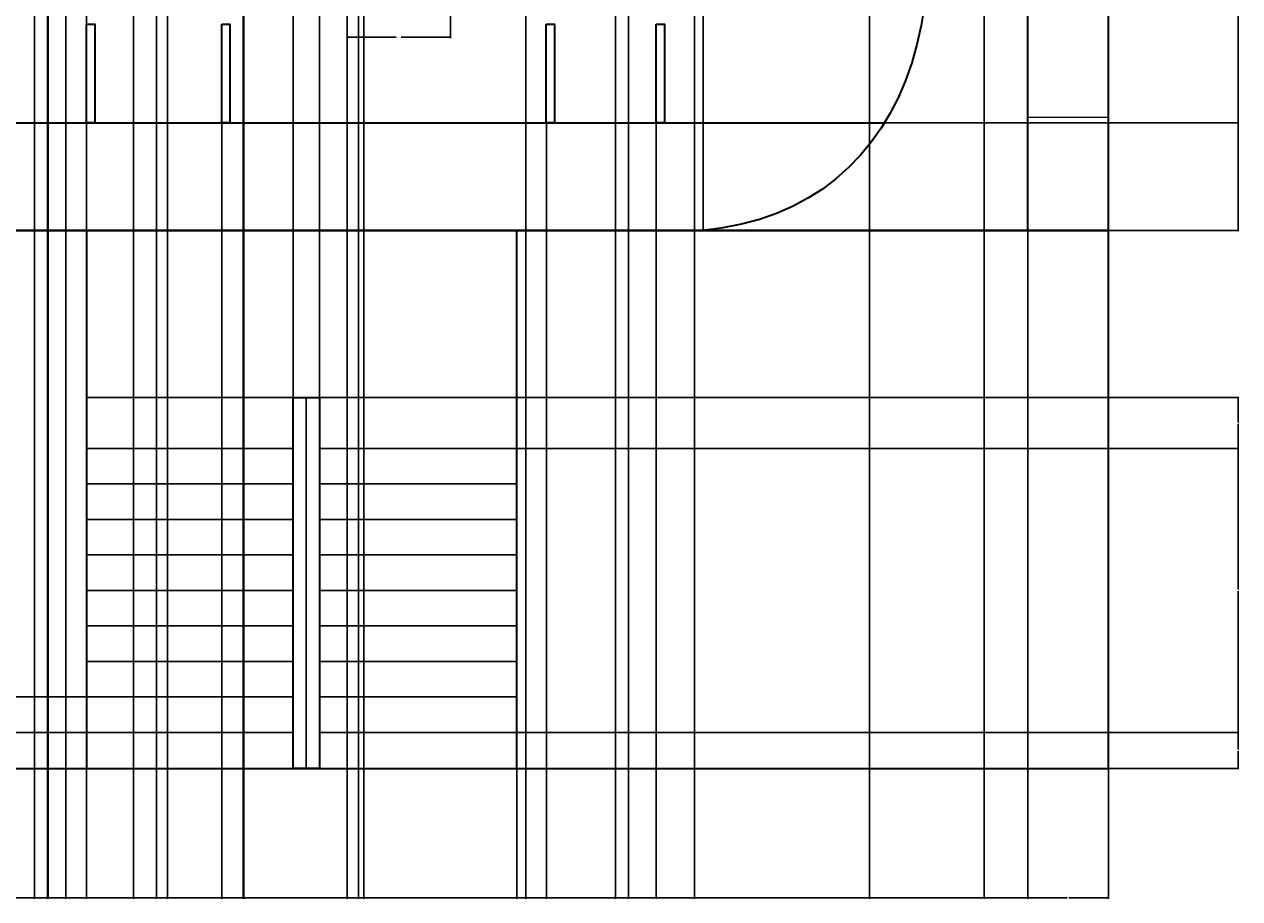
# Model space of a CAD drawing. Units: inches. Extents: x -19 to 408, y -26 to 603.
# Tile 2 of 7: x 137 to 408, y -26 to 169. Entities that reach past the tile are written whole.
import ezdxf

# ---------------------------------------------------------------- set-up
doc = ezdxf.new("R2010")
doc.units = ezdxf.units.IN
doc.header["$MEASUREMENT"] = 0
for name, color, linetype, lineweight in [('A-ANNO-DIMS', 2, 'Continuous', 18), ('A-ELEV', 7, 'Continuous', 35), ('A-FLOR-STRS', 2, 'Continuous', 25), ('A-WALL-PATT', 8, 'Continuous', 13)]:
    doc.layers.add(name, color=color, linetype=linetype, lineweight=lineweight)
doc.styles.get("Standard").update_dxf_attribs({"font": 'arial.ttf'})
doc.dimstyles.get("Standard").update_dxf_attribs({"dimtxt": 0.18, "dimasz": 0.18, "dimexe": 0.18, "dimexo": 0.0625, "dimgap": 0.09, "dimtad": 0, "dimtih": 1, "dimtoh": 1, "dimdec": 4, "dimzin": 0, "dimdsep": 46, "dimtxsty": 'Standard', "dimcen": 0.09, "dimadec": 0, "dimazin": 0, "dimtfac": 1, "dimtdec": 4, "dimtofl": 0, "dimtmove": 0, "dimatfit": 3, "dimfxl": 1, "dimtolj": 1, "dimtzin": 0, "dimarcsym": 0})

# ---------------------------------------------------------------- blocks, each defined once
blk = doc.blocks.new('RAIL-POST')
blk.add_lwpolyline([(0, 22), (1.83, 22), (1.83, 0), (0, 0)], close=True)
blk = doc.blocks.new('*D7')
at = {"layer": 'A-ANNO-DIMS', "color": 0, "lineweight": -2, "transparency": 16777216}
for p, q in [((208.71, 171.08), (208.71, 166.08)), ((231.77, 171.08), (231.77, 166.08)), ((208.89, 166.26), (219.71, 166.26)), ((231.59, 166.26), (220.77, 166.26))]:
    blk.add_line(p, q, dxfattribs=at)
at = {"layer": 'A-ANNO-DIMS', "color": 0, "transparency": 16777216}
for points in [[(208.89, 166.29), (208.89, 166.23), (208.71, 166.26)], [(231.59, 166.29), (231.59, 166.23), (231.77, 166.26)]]:
    blk.add_solid(points, dxfattribs=at)
at = {"layer": 'Defpoints', "color": 0, "transparency": 16777216}
for p in [(208.71, 171.15), (231.77, 171.15), (208.71, 166.26)]:
    blk.add_point(p, dxfattribs=at)
at = {"layer": 'A-ANNO-DIMS', "color": 0, "transparency": 16777216, "insert": (220.24, 166.26), "char_height": 0.18, "attachment_point": 5}
blk.add_mtext('\\A1;23 TYP.', dxfattribs=at)
blk = doc.blocks.new('*D11')
at = {"layer": 'A-ANNO-DIMS', "color": 0, "lineweight": -2, "transparency": 16777216}
for p, q in [((150.57, 123.08), (150.57, -25.93)), ((36.57, 3.08), (36.57, -25.93)), ((36.75, -25.75), (93.29, -25.75)), ((150.39, -25.75), (93.85, -25.75))]:
    blk.add_line(p, q, dxfattribs=at)
at = {"layer": 'A-ANNO-DIMS', "color": 0, "transparency": 16777216}
for points in [[(36.75, -25.72), (36.75, -25.78), (36.57, -25.75)], [(150.39, -25.72), (150.39, -25.78), (150.57, -25.75)]]:
    blk.add_solid(points, dxfattribs=at)
at = {"layer": 'Defpoints', "color": 0, "transparency": 16777216}
for p in [(150.57, 123.15), (36.57, 3.15), (150.57, -25.75)]:
    blk.add_point(p, dxfattribs=at)
at = {"layer": 'A-ANNO-DIMS', "color": 0, "transparency": 16777216, "insert": (93.57, -25.75), "char_height": 0.18, "attachment_point": 5}
blk.add_mtext('\\A1;114', dxfattribs=at)
blk = doc.blocks.new('*D12')
at = {"layer": 'A-ANNO-DIMS', "color": 0, "lineweight": -2, "transparency": 16777216}
for p, q in [((246.57, 123.08), (246.57, -25.93)), ((150.57, 3.08), (150.57, -25.93)), ((150.75, -25.75), (198.35, -25.75)), ((246.39, -25.75), (198.79, -25.75))]:
    blk.add_line(p, q, dxfattribs=at)
at = {"layer": 'A-ANNO-DIMS', "color": 0, "transparency": 16777216}
for points in [[(150.75, -25.72), (150.75, -25.78), (150.57, -25.75)], [(246.39, -25.72), (246.39, -25.78), (246.57, -25.75)]]:
    blk.add_solid(points, dxfattribs=at)
at = {"layer": 'Defpoints', "color": 0, "transparency": 16777216}
for p in [(246.57, 123.15), (150.57, 3.15), (246.57, -25.75)]:
    blk.add_point(p, dxfattribs=at)
at = {"layer": 'A-ANNO-DIMS', "color": 0, "transparency": 16777216, "insert": (198.57, -25.75), "char_height": 0.18, "attachment_point": 5}
blk.add_mtext('\\A1;96', dxfattribs=at)
blk = doc.blocks.new('*D13')
at = {"layer": 'A-ANNO-DIMS', "color": 0, "lineweight": -2, "transparency": 16777216}
for p, q in [((360.57, 123.08), (360.57, -25.93)), ((246.57, 3.08), (246.57, -25.93)), ((246.75, -25.75), (303.29, -25.75)), ((360.39, -25.75), (303.85, -25.75))]:
    blk.add_line(p, q, dxfattribs=at)
at = {"layer": 'A-ANNO-DIMS', "color": 0, "transparency": 16777216}
for points in [[(246.75, -25.72), (246.75, -25.78), (246.57, -25.75)], [(360.39, -25.72), (360.39, -25.78), (360.57, -25.75)]]:
    blk.add_solid(points, dxfattribs=at)
at = {"layer": 'Defpoints', "color": 0, "transparency": 16777216}
for p in [(360.57, 123.15), (246.57, 3.15), (360.57, -25.75)]:
    blk.add_point(p, dxfattribs=at)
at = {"layer": 'A-ANNO-DIMS', "color": 0, "transparency": 16777216, "insert": (303.57, -25.75), "char_height": 0.18, "attachment_point": 5}
blk.add_mtext('\\A1;114', dxfattribs=at)
blk = doc.blocks.new('*D14')
at = {"layer": 'A-ANNO-DIMS', "color": 0, "lineweight": -2, "transparency": 16777216}
for p, q in [((360.57, 123.08), (360.57, -25.93)), ((378.57, 3.08), (378.57, -25.93)), ((360.75, -25.75), (369.36, -25.75)), ((378.39, -25.75), (369.78, -25.75))]:
    blk.add_line(p, q, dxfattribs=at)
at = {"layer": 'A-ANNO-DIMS', "color": 0, "transparency": 16777216}
for points in [[(360.75, -25.72), (360.75, -25.78), (360.57, -25.75)], [(378.39, -25.72), (378.39, -25.78), (378.57, -25.75)]]:
    blk.add_solid(points, dxfattribs=at)
at = {"layer": 'Defpoints', "color": 0, "transparency": 16777216}
for p in [(360.57, 123.15), (378.57, 3.15), (378.57, -25.75)]:
    blk.add_point(p, dxfattribs=at)
at = {"layer": 'A-ANNO-DIMS', "color": 0, "transparency": 16777216, "insert": (369.57, -25.75), "char_height": 0.18, "attachment_point": 5}
blk.add_mtext('\\A1;18', dxfattribs=at)
blk = doc.blocks.new('*D23')
at = {"layer": 'A-ANNO-DIMS', "color": 0, "lineweight": -2, "transparency": 16777216}
for p, q in [((360.63, 411.15), (407.65, 411.15)), ((407.47, 410.97), (407.47, 267.33)), ((407.47, 123.33), (407.47, 266.97)), ((360.63, 123.15), (407.65, 123.15))]:
    blk.add_line(p, q, dxfattribs=at)
at = {"layer": 'A-ANNO-DIMS', "color": 0, "transparency": 16777216}
for points in [[(407.44, 410.97), (407.5, 410.97), (407.47, 411.15)], [(407.44, 123.33), (407.5, 123.33), (407.47, 123.15)]]:
    blk.add_solid(points, dxfattribs=at)
at = {"layer": 'Defpoints', "color": 0, "transparency": 16777216}
for p in [(360.57, 411.15), (407.47, 411.15), (360.57, 123.15)]:
    blk.add_point(p, dxfattribs=at)
at = {"layer": 'A-ANNO-DIMS', "color": 0, "transparency": 16777216, "insert": (407.47, 267.15), "char_height": 0.18, "attachment_point": 5}
blk.add_mtext('\\A1;288', dxfattribs=at)
blk = doc.blocks.new('*D27')
at = {"layer": 'A-ANNO-DIMS', "color": 0, "lineweight": -2, "transparency": 16777216}
for p, q in [((288.17, 123.21), (288.17, 602.9)), ((288.35, 602.72), (324.05, 602.72)), ((360.39, 602.72), (324.69, 602.72)), ((360.57, 123.21), (360.57, 602.9))]:
    blk.add_line(p, q, dxfattribs=at)
at = {"layer": 'A-ANNO-DIMS', "color": 0, "transparency": 16777216}
for points in [[(288.35, 602.75), (288.35, 602.69), (288.17, 602.72)], [(360.39, 602.75), (360.39, 602.69), (360.57, 602.72)]]:
    blk.add_solid(points, dxfattribs=at)
at = {"layer": 'Defpoints', "color": 0, "transparency": 16777216}
for p in [(360.57, 602.72), (288.17, 123.15), (360.57, 123.15)]:
    blk.add_point(p, dxfattribs=at)
at = {"layer": 'A-ANNO-DIMS', "color": 0, "transparency": 16777216, "insert": (324.37, 602.72), "char_height": 0.18, "attachment_point": 5}
blk.add_mtext('\\A1;72.4', dxfattribs=at)
blk = doc.blocks.new('*D30')
at = {"layer": 'A-ANNO-DIMS', "color": 0, "lineweight": -2, "transparency": 16777216}
for p, q in [((360.57, 411.08), (360.57, -25.93)), ((185.52, 387.08), (185.52, -25.93)), ((185.7, -25.75), (272.59, -25.75)), ((360.39, -25.75), (273.5, -25.75))]:
    blk.add_line(p, q, dxfattribs=at)
at = {"layer": 'A-ANNO-DIMS', "color": 0, "transparency": 16777216}
for points in [[(185.7, -25.72), (185.7, -25.78), (185.52, -25.75)], [(360.39, -25.72), (360.39, -25.78), (360.57, -25.75)]]:
    blk.add_solid(points, dxfattribs=at)
at = {"layer": 'Defpoints', "color": 0, "transparency": 16777216}
for p in [(360.57, 411.15), (185.52, 387.15), (360.57, -25.75)]:
    blk.add_point(p, dxfattribs=at)
at = {"layer": 'A-ANNO-DIMS', "color": 0, "transparency": 16777216, "insert": (273.05, -25.75), "char_height": 0.18, "attachment_point": 5}
blk.add_mtext('\\A1;175.05', dxfattribs=at)
blk = doc.blocks.new('*D32')
at = {"layer": 'A-ANNO-DIMS', "color": 0, "lineweight": -2, "transparency": 16777216}
for p, q in [((328.66, 147.15), (407.65, 147.15)), ((407.47, 146.97), (407.47, 135.33)), ((407.47, 123.33), (407.47, 134.97)), ((288.23, 123.15), (407.65, 123.15))]:
    blk.add_line(p, q, dxfattribs=at)
at = {"layer": 'A-ANNO-DIMS', "color": 0, "transparency": 16777216}
for points in [[(407.44, 146.97), (407.5, 146.97), (407.47, 147.15)], [(407.44, 123.33), (407.5, 123.33), (407.47, 123.15)]]:
    blk.add_solid(points, dxfattribs=at)
at = {"layer": 'Defpoints', "color": 0, "transparency": 16777216}
for p in [(328.59, 147.15), (407.47, 147.15), (288.17, 123.15)]:
    blk.add_point(p, dxfattribs=at)
at = {"layer": 'A-ANNO-DIMS', "color": 0, "transparency": 16777216, "insert": (407.47, 135.15), "char_height": 0.18, "attachment_point": 5}
blk.add_mtext('\\A1;24', dxfattribs=at)
blk = doc.blocks.new('*D41')
at = {"layer": 'A-ANNO-DIMS', "color": 0, "lineweight": -2, "transparency": 16777216}
for p, q in [((87.25, 147.08), (87.25, -25.93)), ((150.62, 147.08), (150.62, -25.93)), ((87.43, -25.75), (118.54, -25.75)), ((150.44, -25.75), (119.33, -25.75))]:
    blk.add_line(p, q, dxfattribs=at)
at = {"layer": 'A-ANNO-DIMS', "color": 0, "transparency": 16777216}
for points in [[(87.43, -25.72), (87.43, -25.78), (87.25, -25.75)], [(150.44, -25.72), (150.44, -25.78), (150.62, -25.75)]]:
    blk.add_solid(points, dxfattribs=at)
at = {"layer": 'Defpoints', "color": 0, "transparency": 16777216}
for p in [(87.25, 147.15), (150.62, 147.15), (150.62, -25.75)]:
    blk.add_point(p, dxfattribs=at)
at = {"layer": 'A-ANNO-DIMS', "color": 0, "transparency": 16777216, "insert": (118.93, -25.75), "char_height": 0.18, "attachment_point": 5}
blk.add_mtext('\\A1;63.36', dxfattribs=at)
blk = doc.blocks.new('*D42')
at = {"layer": 'A-ANNO-DIMS', "color": 0, "lineweight": -2, "transparency": 16777216}
for p, q in [((150.62, 147.08), (150.62, -25.93)), ((180.76, 147.08), (180.76, -25.93)), ((150.8, -25.75), (165.29, -25.75)), ((180.58, -25.75), (166.08, -25.75))]:
    blk.add_line(p, q, dxfattribs=at)
at = {"layer": 'A-ANNO-DIMS', "color": 0, "transparency": 16777216}
for points in [[(150.8, -25.72), (150.8, -25.78), (150.62, -25.75)], [(180.58, -25.72), (180.58, -25.78), (180.76, -25.75)]]:
    blk.add_solid(points, dxfattribs=at)
at = {"layer": 'Defpoints', "color": 0, "transparency": 16777216}
for p in [(150.62, 147.15), (180.76, 147.15), (180.76, -25.75)]:
    blk.add_point(p, dxfattribs=at)
at = {"layer": 'A-ANNO-DIMS', "color": 0, "transparency": 16777216, "insert": (165.69, -25.75), "char_height": 0.18, "attachment_point": 5}
blk.add_mtext('\\A1;30.14', dxfattribs=at)
blk = doc.blocks.new('*D43')
at = {"layer": 'A-ANNO-DIMS', "color": 0, "lineweight": -2, "transparency": 16777216}
for p, q in [((180.76, 147.08), (180.76, -25.93)), ((253.18, 147.08), (253.18, -25.93)), ((180.94, -25.75), (216.57, -25.75)), ((253, -25.75), (217.36, -25.75))]:
    blk.add_line(p, q, dxfattribs=at)
at = {"layer": 'A-ANNO-DIMS', "color": 0, "transparency": 16777216}
for points in [[(180.94, -25.72), (180.94, -25.78), (180.76, -25.75)], [(253, -25.72), (253, -25.78), (253.18, -25.75)]]:
    blk.add_solid(points, dxfattribs=at)
at = {"layer": 'Defpoints', "color": 0, "transparency": 16777216}
for p in [(180.76, 147.15), (253.18, 147.15), (253.18, -25.75)]:
    blk.add_point(p, dxfattribs=at)
at = {"layer": 'A-ANNO-DIMS', "color": 0, "transparency": 16777216, "insert": (216.97, -25.75), "char_height": 0.18, "attachment_point": 5}
blk.add_mtext('\\A1;72.42', dxfattribs=at)
blk = doc.blocks.new('*D44')
at = {"layer": 'A-ANNO-DIMS', "color": 0, "lineweight": -2, "transparency": 16777216}
for p, q in [((253.18, 147.08), (253.18, -25.93)), ((277.69, 147.08), (277.69, -25.93)), ((253.36, -25.75), (265.05, -25.75)), ((277.51, -25.75), (265.81, -25.75))]:
    blk.add_line(p, q, dxfattribs=at)
at = {"layer": 'A-ANNO-DIMS', "color": 0, "transparency": 16777216}
for points in [[(253.36, -25.72), (253.36, -25.78), (253.18, -25.75)], [(277.51, -25.72), (277.51, -25.78), (277.69, -25.75)]]:
    blk.add_solid(points, dxfattribs=at)
at = {"layer": 'Defpoints', "color": 0, "transparency": 16777216}
for p in [(253.18, 147.15), (277.69, 147.15), (277.69, -25.75)]:
    blk.add_point(p, dxfattribs=at)
at = {"layer": 'A-ANNO-DIMS', "color": 0, "transparency": 16777216, "insert": (265.43, -25.75), "char_height": 0.18, "attachment_point": 5}
blk.add_mtext('\\A1;24.51', dxfattribs=at)
blk = doc.blocks.new('*D53')
at = {"layer": 'A-ANNO-DIMS', "color": 0, "lineweight": -2, "transparency": 16777216}
for p, q in [((142.02, 171.08), (142.02, -25.93)), ((146.02, 171.08), (146.02, -25.93)), ((142.2, -25.75), (143.87, -25.75)), ((145.84, -25.75), (144.18, -25.75))]:
    blk.add_line(p, q, dxfattribs=at)
at = {"layer": 'A-ANNO-DIMS', "color": 0, "transparency": 16777216}
for points in [[(142.2, -25.72), (142.2, -25.78), (142.02, -25.75)], [(145.84, -25.72), (145.84, -25.78), (146.02, -25.75)]]:
    blk.add_solid(points, dxfattribs=at)
at = {"layer": 'Defpoints', "color": 0, "transparency": 16777216}
for p in [(142.02, 171.15), (146.02, 171.15), (146.02, -25.75)]:
    blk.add_point(p, dxfattribs=at)
at = {"layer": 'A-ANNO-DIMS', "color": 0, "transparency": 16777216, "insert": (144.02, -25.75), "char_height": 0.18, "attachment_point": 5}
blk.add_mtext('\\A1;4', dxfattribs=at)
blk = doc.blocks.new('*D54')
at = {"layer": 'A-ANNO-DIMS', "color": 0, "lineweight": -2, "transparency": 16777216}
for p, q in [((146.02, 171.08), (146.02, -25.93)), ((161.09, 171.08), (161.09, -25.93)), ((146.2, -25.75), (153.1, -25.75)), ((160.91, -25.75), (154.01, -25.75))]:
    blk.add_line(p, q, dxfattribs=at)
at = {"layer": 'A-ANNO-DIMS', "color": 0, "transparency": 16777216}
for points in [[(146.2, -25.72), (146.2, -25.78), (146.02, -25.75)], [(160.91, -25.72), (160.91, -25.78), (161.09, -25.75)]]:
    blk.add_solid(points, dxfattribs=at)
at = {"layer": 'Defpoints', "color": 0, "transparency": 16777216}
for p in [(146.02, 171.15), (161.09, 171.15), (161.09, -25.75)]:
    blk.add_point(p, dxfattribs=at)
at = {"layer": 'A-ANNO-DIMS', "color": 0, "transparency": 16777216, "insert": (153.56, -25.75), "char_height": 0.18, "attachment_point": 5}
blk.add_mtext('\\A1;15.064', dxfattribs=at)
blk = doc.blocks.new('*D62')
at = {"layer": 'A-ANNO-DIMS', "color": 0, "lineweight": -2, "transparency": 16777216}
for p, q in [((131.96, 267.08), (131.96, -25.93)), ((185.68, 267.08), (185.68, -25.93)), ((132.14, -25.75), (158.43, -25.75)), ((185.5, -25.75), (159.21, -25.75))]:
    blk.add_line(p, q, dxfattribs=at)
at = {"layer": 'A-ANNO-DIMS', "color": 0, "transparency": 16777216}
for points in [[(132.14, -25.72), (132.14, -25.78), (131.96, -25.75)], [(185.5, -25.72), (185.5, -25.78), (185.68, -25.75)]]:
    blk.add_solid(points, dxfattribs=at)
at = {"layer": 'Defpoints', "color": 0, "transparency": 16777216}
for p in [(131.96, 267.15), (185.68, 267.15), (185.68, -25.75)]:
    blk.add_point(p, dxfattribs=at)
at = {"layer": 'A-ANNO-DIMS', "color": 0, "transparency": 16777216, "insert": (158.82, -25.75), "char_height": 0.18, "attachment_point": 5}
blk.add_mtext('\\A1;53.72', dxfattribs=at)
blk = doc.blocks.new('*D63')
at = {"layer": 'A-ANNO-DIMS', "color": 0, "lineweight": -2, "transparency": 16777216}
for p, q in [((185.68, 267.08), (185.68, -25.93)), ((211.27, 267.08), (211.27, -25.93)), ((185.86, -25.75), (198.01, -25.75)), ((211.09, -25.75), (198.94, -25.75))]:
    blk.add_line(p, q, dxfattribs=at)
at = {"layer": 'A-ANNO-DIMS', "color": 0, "transparency": 16777216}
for points in [[(185.86, -25.72), (185.86, -25.78), (185.68, -25.75)], [(211.09, -25.72), (211.09, -25.78), (211.27, -25.75)]]:
    blk.add_solid(points, dxfattribs=at)
at = {"layer": 'Defpoints', "color": 0, "transparency": 16777216}
for p in [(185.68, 267.15), (211.27, 267.15), (211.27, -25.75)]:
    blk.add_point(p, dxfattribs=at)
at = {"layer": 'A-ANNO-DIMS', "color": 0, "transparency": 16777216, "insert": (198.47, -25.75), "char_height": 0.18, "attachment_point": 5}
blk.add_mtext('\\A1;25.584', dxfattribs=at)
blk = doc.blocks.new('*D64')
at = {"layer": 'A-ANNO-DIMS', "color": 0, "lineweight": -2, "transparency": 16777216}
for p, q in [((211.27, 267.08), (211.27, -25.93)), ((268.61, 267.08), (268.61, -25.93)), ((211.45, -25.75), (239.55, -25.75)), ((268.43, -25.75), (240.33, -25.75))]:
    blk.add_line(p, q, dxfattribs=at)
at = {"layer": 'A-ANNO-DIMS', "color": 0, "transparency": 16777216}
for points in [[(211.45, -25.72), (211.45, -25.78), (211.27, -25.75)], [(268.43, -25.72), (268.43, -25.78), (268.61, -25.75)]]:
    blk.add_solid(points, dxfattribs=at)
at = {"layer": 'Defpoints', "color": 0, "transparency": 16777216}
for p in [(211.27, 267.15), (268.61, 267.15), (268.61, -25.75)]:
    blk.add_point(p, dxfattribs=at)
at = {"layer": 'A-ANNO-DIMS', "color": 0, "transparency": 16777216, "insert": (239.94, -25.75), "char_height": 0.18, "attachment_point": 5}
blk.add_mtext('\\A1;57.34', dxfattribs=at)
blk = doc.blocks.new('*D65')
at = {"layer": 'A-ANNO-DIMS', "color": 0, "lineweight": -2, "transparency": 16777216}
for p, q in [((268.61, 267.08), (268.61, -25.93)), ((286.26, 267.08), (286.26, -25.93)), ((268.79, -25.75), (276.98, -25.75)), ((286.08, -25.75), (277.89, -25.75))]:
    blk.add_line(p, q, dxfattribs=at)
at = {"layer": 'A-ANNO-DIMS', "color": 0, "transparency": 16777216}
for points in [[(268.79, -25.72), (268.79, -25.78), (268.61, -25.75)], [(286.08, -25.72), (286.08, -25.78), (286.26, -25.75)]]:
    blk.add_solid(points, dxfattribs=at)
at = {"layer": 'Defpoints', "color": 0, "transparency": 16777216}
for p in [(268.61, 267.15), (286.26, 267.15), (286.26, -25.75)]:
    blk.add_point(p, dxfattribs=at)
at = {"layer": 'A-ANNO-DIMS', "color": 0, "transparency": 16777216, "insert": (277.43, -25.75), "char_height": 0.18, "attachment_point": 5}
blk.add_mtext('\\A1;17.644', dxfattribs=at)
blk = doc.blocks.new('*D70')
at = {"layer": 'A-ANNO-DIMS', "color": 0, "lineweight": -2, "transparency": 16777216}
for p, q in [((150.62, 387.08), (150.62, -25.93)), ((185.52, 387.08), (185.52, -25.93)), ((150.8, -25.75), (167.6, -25.75)), ((185.34, -25.75), (168.53, -25.75))]:
    blk.add_line(p, q, dxfattribs=at)
at = {"layer": 'A-ANNO-DIMS', "color": 0, "transparency": 16777216}
for points in [[(150.8, -25.72), (150.8, -25.78), (150.62, -25.75)], [(185.34, -25.72), (185.34, -25.78), (185.52, -25.75)]]:
    blk.add_solid(points, dxfattribs=at)
at = {"layer": 'Defpoints', "color": 0, "transparency": 16777216}
for p in [(150.62, 387.15), (185.52, 387.15), (185.52, -25.75)]:
    blk.add_point(p, dxfattribs=at)
at = {"layer": 'A-ANNO-DIMS', "color": 0, "transparency": 16777216, "insert": (168.07, -25.75), "char_height": 0.18, "attachment_point": 5}
blk.add_mtext('\\A1;34.906', dxfattribs=at)
blk = doc.blocks.new('*D73')
at = {"layer": 'A-ANNO-DIMS', "color": 0, "lineweight": -2, "transparency": 16777216}
for p, q in [((185.52, 411.08), (185.52, -25.93)), ((208.71, 411.08), (208.71, -25.93)), ((185.7, -25.75), (196.72, -25.75)), ((208.53, -25.75), (197.51, -25.75))]:
    blk.add_line(p, q, dxfattribs=at)
at = {"layer": 'A-ANNO-DIMS', "color": 0, "transparency": 16777216}
for points in [[(185.7, -25.72), (185.7, -25.78), (185.52, -25.75)], [(208.53, -25.72), (208.53, -25.78), (208.71, -25.75)]]:
    blk.add_solid(points, dxfattribs=at)
at = {"layer": 'Defpoints', "color": 0, "transparency": 16777216}
for p in [(185.52, 411.15), (208.71, 411.15), (208.71, -25.75)]:
    blk.add_point(p, dxfattribs=at)
at = {"layer": 'A-ANNO-DIMS', "color": 0, "transparency": 16777216, "insert": (197.12, -25.75), "char_height": 0.18, "attachment_point": 5}
blk.add_mtext('\\A1;23.19', dxfattribs=at)
blk = doc.blocks.new('*D75')
at = {"layer": 'A-ANNO-DIMS', "color": 0, "lineweight": -2, "transparency": 16777216}
for p, q in [((212.43, 507.08), (212.43, -25.93)), ((248.57, 507.08), (248.57, -25.93)), ((212.61, -25.75), (230.11, -25.75)), ((248.39, -25.75), (230.89, -25.75))]:
    blk.add_line(p, q, dxfattribs=at)
at = {"layer": 'A-ANNO-DIMS', "color": 0, "transparency": 16777216}
for points in [[(212.61, -25.72), (212.61, -25.78), (212.43, -25.75)], [(248.39, -25.72), (248.39, -25.78), (248.57, -25.75)]]:
    blk.add_solid(points, dxfattribs=at)
at = {"layer": 'Defpoints', "color": 0, "transparency": 16777216}
for p in [(212.43, 507.15), (248.57, 507.15), (248.57, -25.75)]:
    blk.add_point(p, dxfattribs=at)
at = {"layer": 'A-ANNO-DIMS', "color": 0, "transparency": 16777216, "insert": (230.5, -25.75), "char_height": 0.18, "attachment_point": 5}
blk.add_mtext('\\A1;36.14', dxfattribs=at)
blk = doc.blocks.new('*D76')
at = {"layer": 'A-ANNO-DIMS', "color": 0, "lineweight": -2, "transparency": 16777216}
for p, q in [((248.57, 507.08), (248.57, -25.93)), ((271.51, 507.08), (271.51, -25.93)), ((248.75, -25.75), (259.58, -25.75)), ((271.33, -25.75), (260.51, -25.75))]:
    blk.add_line(p, q, dxfattribs=at)
at = {"layer": 'A-ANNO-DIMS', "color": 0, "transparency": 16777216}
for points in [[(248.75, -25.72), (248.75, -25.78), (248.57, -25.75)], [(271.33, -25.72), (271.33, -25.78), (271.51, -25.75)]]:
    blk.add_solid(points, dxfattribs=at)
at = {"layer": 'Defpoints', "color": 0, "transparency": 16777216}
for p in [(248.57, 507.15), (271.51, 507.15), (271.51, -25.75)]:
    blk.add_point(p, dxfattribs=at)
at = {"layer": 'A-ANNO-DIMS', "color": 0, "transparency": 16777216, "insert": (260.04, -25.75), "char_height": 0.18, "attachment_point": 5}
blk.add_mtext('\\A1;22.944', dxfattribs=at)
blk = doc.blocks.new('*D77')
at = {"layer": 'A-ANNO-DIMS', "color": 0, "lineweight": -2, "transparency": 16777216}
for p, q in [((271.51, 507.08), (271.51, -25.93)), ((325.24, 507.08), (325.24, -25.93)), ((271.69, -25.75), (297.98, -25.75)), ((325.06, -25.75), (298.77, -25.75))]:
    blk.add_line(p, q, dxfattribs=at)
at = {"layer": 'A-ANNO-DIMS', "color": 0, "transparency": 16777216}
for points in [[(271.69, -25.72), (271.69, -25.78), (271.51, -25.75)], [(325.06, -25.72), (325.06, -25.78), (325.24, -25.75)]]:
    blk.add_solid(points, dxfattribs=at)
at = {"layer": 'Defpoints', "color": 0, "transparency": 16777216}
for p in [(271.51, 507.15), (325.24, 507.15), (325.24, -25.75)]:
    blk.add_point(p, dxfattribs=at)
at = {"layer": 'A-ANNO-DIMS', "color": 0, "transparency": 16777216, "insert": (298.38, -25.75), "char_height": 0.18, "attachment_point": 5}
blk.add_mtext('\\A1;53.72', dxfattribs=at)
blk = doc.blocks.new('*D78')
at = {"layer": 'A-ANNO-DIMS', "color": 0, "lineweight": -2, "transparency": 16777216}
for p, q in [((325.24, 507.08), (325.24, -25.93)), ((350.82, 507.08), (350.82, -25.93)), ((325.42, -25.75), (337.56, -25.75)), ((350.64, -25.75), (338.49, -25.75))]:
    blk.add_line(p, q, dxfattribs=at)
at = {"layer": 'A-ANNO-DIMS', "color": 0, "transparency": 16777216}
for points in [[(325.42, -25.72), (325.42, -25.78), (325.24, -25.75)], [(350.64, -25.72), (350.64, -25.78), (350.82, -25.75)]]:
    blk.add_solid(points, dxfattribs=at)
at = {"layer": 'Defpoints', "color": 0, "transparency": 16777216}
for p in [(325.24, 507.15), (350.82, 507.15), (350.82, -25.75)]:
    blk.add_point(p, dxfattribs=at)
at = {"layer": 'A-ANNO-DIMS', "color": 0, "transparency": 16777216, "insert": (338.03, -25.75), "char_height": 0.18, "attachment_point": 5}
blk.add_mtext('\\A1;25.584', dxfattribs=at)
blk = doc.blocks.new('*D83')
at = {"layer": 'A-ANNO-DIMS', "color": 0, "lineweight": -2, "transparency": 16777216}
for p, q in [((141.92, 491.44), (141.92, -25.93)), ((166.23, 491.44), (166.23, -25.93)), ((142.1, -25.75), (153.69, -25.75)), ((166.05, -25.75), (154.45, -25.75))]:
    blk.add_line(p, q, dxfattribs=at)
at = {"layer": 'A-ANNO-DIMS', "color": 0, "transparency": 16777216}
for points in [[(142.1, -25.72), (142.1, -25.78), (141.92, -25.75)], [(166.05, -25.72), (166.05, -25.78), (166.23, -25.75)]]:
    blk.add_solid(points, dxfattribs=at)
at = {"layer": 'Defpoints', "color": 0, "transparency": 16777216}
for p in [(141.92, 491.5), (166.23, 491.5), (166.23, -25.75)]:
    blk.add_point(p, dxfattribs=at)
at = {"layer": 'A-ANNO-DIMS', "color": 0, "transparency": 16777216, "insert": (154.07, -25.75), "char_height": 0.18, "attachment_point": 5}
blk.add_mtext('\\A1;24.31', dxfattribs=at)
blk = doc.blocks.new('*D84')
at = {"layer": 'A-ANNO-DIMS', "color": 0, "lineweight": -2, "transparency": 16777216}
for p, q in [((138.97, 531.28), (138.97, -25.93)), ((168.64, 531.28), (168.64, -25.93)), ((139.15, -25.75), (153.41, -25.75)), ((168.46, -25.75), (154.2, -25.75))]:
    blk.add_line(p, q, dxfattribs=at)
at = {"layer": 'A-ANNO-DIMS', "color": 0, "transparency": 16777216}
for points in [[(139.15, -25.72), (139.15, -25.78), (138.97, -25.75)], [(168.46, -25.72), (168.46, -25.78), (168.64, -25.75)]]:
    blk.add_solid(points, dxfattribs=at)
at = {"layer": 'Defpoints', "color": 0, "transparency": 16777216}
for p in [(138.97, 531.34), (168.64, 531.34), (168.64, -25.75)]:
    blk.add_point(p, dxfattribs=at)
at = {"layer": 'A-ANNO-DIMS', "color": 0, "transparency": 16777216, "insert": (153.81, -25.75), "char_height": 0.18, "attachment_point": 5}
blk.add_mtext('\\A1;29.67', dxfattribs=at)
blk = doc.blocks.new('*D91')
at = {"layer": 'A-ANNO-DIMS', "color": 0, "lineweight": -2, "transparency": 16777216}
for p, q in [((246.63, 11.18), (407.65, 11.18)), ((407.47, 11), (407.47, 7.35)), ((407.47, 3.33), (407.47, 6.98)), ((246.63, 3.15), (407.65, 3.15))]:
    blk.add_line(p, q, dxfattribs=at)
at = {"layer": 'A-ANNO-DIMS', "color": 0, "transparency": 16777216}
for points in [[(407.44, 11), (407.5, 11), (407.47, 11.18)], [(407.44, 3.33), (407.5, 3.33), (407.47, 3.15)]]:
    blk.add_solid(points, dxfattribs=at)
at = {"layer": 'Defpoints', "color": 0, "transparency": 16777216}
for p in [(246.57, 11.18), (407.47, 11.18), (246.57, 3.15)]:
    blk.add_point(p, dxfattribs=at)
at = {"layer": 'A-ANNO-DIMS', "color": 0, "transparency": 16777216, "insert": (407.47, 7.17), "char_height": 0.18, "attachment_point": 5}
blk.add_mtext('\\A1;8.036', dxfattribs=at)
blk = doc.blocks.new('*D92')
at = {"layer": 'A-ANNO-DIMS', "color": 0, "lineweight": -2, "transparency": 16777216}
for p, q in [((246.63, 74.54), (407.65, 74.54)), ((407.47, 74.36), (407.47, 43.04)), ((407.47, 11.36), (407.47, 42.68)), ((246.63, 11.18), (407.65, 11.18))]:
    blk.add_line(p, q, dxfattribs=at)
at = {"layer": 'A-ANNO-DIMS', "color": 0, "transparency": 16777216}
for points in [[(407.44, 74.36), (407.5, 74.36), (407.47, 74.54)], [(407.44, 11.36), (407.5, 11.36), (407.47, 11.18)]]:
    blk.add_solid(points, dxfattribs=at)
at = {"layer": 'Defpoints', "color": 0, "transparency": 16777216}
for p in [(246.57, 74.54), (407.47, 74.54), (246.57, 11.18)]:
    blk.add_point(p, dxfattribs=at)
at = {"layer": 'A-ANNO-DIMS', "color": 0, "transparency": 16777216, "insert": (407.47, 42.86), "char_height": 0.18, "attachment_point": 5}
blk.add_mtext('\\A1;63.35', dxfattribs=at)
blk = doc.blocks.new('*D93')
at = {"layer": 'A-ANNO-DIMS', "color": 0, "lineweight": -2, "transparency": 16777216}
for p, q in [((246.63, 85.9), (407.65, 85.9)), ((407.47, 85.72), (407.47, 80.4)), ((407.47, 74.72), (407.47, 80.04)), ((246.63, 74.54), (407.65, 74.54))]:
    blk.add_line(p, q, dxfattribs=at)
at = {"layer": 'A-ANNO-DIMS', "color": 0, "transparency": 16777216}
for points in [[(407.44, 85.72), (407.5, 85.72), (407.47, 85.9)], [(407.44, 74.72), (407.5, 74.72), (407.47, 74.54)]]:
    blk.add_solid(points, dxfattribs=at)
at = {"layer": 'Defpoints', "color": 0, "transparency": 16777216}
for p in [(246.57, 85.9), (407.47, 85.9), (246.57, 74.54)]:
    blk.add_point(p, dxfattribs=at)
at = {"layer": 'A-ANNO-DIMS', "color": 0, "transparency": 16777216, "insert": (407.47, 80.22), "char_height": 0.18, "attachment_point": 5}
blk.add_mtext('\\A1;11.368', dxfattribs=at)
blk = doc.blocks.new('*D94')
at = {"layer": 'A-ANNO-DIMS', "color": 0, "lineweight": -2, "transparency": 16777216}
for p, q in [((150.51, 19.1), (-18.88, 19.1)), ((-18.7, 18.92), (-18.7, 15.32)), ((-18.7, 11.36), (-18.7, 14.96)), ((150.51, 11.18), (-18.88, 11.18))]:
    blk.add_line(p, q, dxfattribs=at)
at = {"layer": 'A-ANNO-DIMS', "color": 0, "transparency": 16777216}
for points in [[(-18.73, 18.92), (-18.67, 18.92), (-18.7, 19.1)], [(-18.73, 11.36), (-18.67, 11.36), (-18.7, 11.18)]]:
    blk.add_solid(points, dxfattribs=at)
at = {"layer": 'Defpoints', "color": 0, "transparency": 16777216}
for p in [(-18.7, 19.1), (150.57, 19.1), (150.57, 11.18)]:
    blk.add_point(p, dxfattribs=at)
at = {"layer": 'A-ANNO-DIMS', "color": 0, "transparency": 16777216, "insert": (-18.7, 15.14), "char_height": 0.18, "attachment_point": 5}
blk.add_mtext('\\A1;7.919', dxfattribs=at)
blk = doc.blocks.new('*D95')
at = {"layer": 'A-ANNO-DIMS', "color": 0, "lineweight": -2, "transparency": 16777216}
for p, q in [((150.57, 85.97), (150.57, 602.9)), ((150.75, 602.72), (173.31, 602.72)), ((196.49, 602.72), (173.93, 602.72)), ((196.67, 85.97), (196.67, 602.9))]:
    blk.add_line(p, q, dxfattribs=at)
at = {"layer": 'A-ANNO-DIMS', "color": 0, "transparency": 16777216}
for points in [[(150.75, 602.75), (150.75, 602.69), (150.57, 602.72)], [(196.49, 602.75), (196.49, 602.69), (196.67, 602.72)]]:
    blk.add_solid(points, dxfattribs=at)
at = {"layer": 'Defpoints', "color": 0, "transparency": 16777216}
for p in [(196.67, 602.72), (150.57, 85.9), (196.67, 85.9)]:
    blk.add_point(p, dxfattribs=at)
at = {"layer": 'A-ANNO-DIMS', "color": 0, "transparency": 16777216, "insert": (173.62, 602.72), "char_height": 0.18, "attachment_point": 5}
blk.add_mtext('\\A1;46.1', dxfattribs=at)
blk = doc.blocks.new('*D96')
at = {"layer": 'A-ANNO-DIMS', "color": 0, "lineweight": -2, "transparency": 16777216}
for p, q in [((196.67, 85.97), (196.67, 602.9)), ((196.85, 602.72), (199.31, 602.72)), ((202.41, 602.72), (199.96, 602.72)), ((202.59, 85.97), (202.59, 602.9))]:
    blk.add_line(p, q, dxfattribs=at)
at = {"layer": 'A-ANNO-DIMS', "color": 0, "transparency": 16777216}
for points in [[(196.85, 602.75), (196.85, 602.69), (196.67, 602.72)], [(202.41, 602.75), (202.41, 602.69), (202.59, 602.72)]]:
    blk.add_solid(points, dxfattribs=at)
at = {"layer": 'Defpoints', "color": 0, "transparency": 16777216}
for p in [(202.59, 602.72), (196.67, 85.9), (202.59, 85.9)]:
    blk.add_point(p, dxfattribs=at)
at = {"layer": 'A-ANNO-DIMS', "color": 0, "transparency": 16777216, "insert": (199.63, 602.72), "char_height": 0.18, "attachment_point": 5}
blk.add_mtext('\\A1;5.92', dxfattribs=at)
blk = doc.blocks.new('*D106')
at = {"layer": 'A-ANNO-DIMS', "color": 0, "lineweight": -2, "transparency": 16777216}
for p, q in [((106.54, 387.08), (106.54, -25.93)), ((185.52, 387.08), (185.52, -25.93)), ((106.72, -25.75), (145.64, -25.75)), ((185.34, -25.75), (146.43, -25.75))]:
    blk.add_line(p, q, dxfattribs=at)
at = {"layer": 'A-ANNO-DIMS', "color": 0, "transparency": 16777216}
for points in [[(106.72, -25.72), (106.72, -25.78), (106.54, -25.75)], [(185.34, -25.72), (185.34, -25.78), (185.52, -25.75)]]:
    blk.add_solid(points, dxfattribs=at)
at = {"layer": 'Defpoints', "color": 0, "transparency": 16777216}
for p in [(106.54, 387.15), (185.52, 387.15), (106.54, -25.75)]:
    blk.add_point(p, dxfattribs=at)
at = {"layer": 'A-ANNO-DIMS', "color": 0, "transparency": 16777216, "insert": (146.03, -25.75), "char_height": 0.18, "attachment_point": 5}
blk.add_mtext('\\A1;78.98', dxfattribs=at)

msp = doc.modelspace()

# ---------------------------------------------------------------- linework, layer by layer
at = {"layer": 'A-ELEV'}
for p, q in [((360.5712, 123.1472), (360.5712, 483.1472)), ((378.5712, 123.1472), (378.5712, 483.1472)), ((36.5712, 147.1472), (328.594, 147.1472)), ((378.5712, 123.1472), (18.5712, 123.1472)), ((18.5712, 123.1472), (378.5712, 123.1472)), ((150.5712, 123.1472), (150.5712, 3.1472)), ((246.5712, 3.1472), (246.5712, 123.1472)), ((378.5712, 3.1472), (378.5712, 123.1472)), ((18.5712, 3.1472), (378.5712, 3.1472))]:
    msp.add_line(p, q, dxfattribs=at)
msp.add_lwpolyline([(196.6731, 85.9033), (202.5934, 85.9033), (202.5934, 3.1472), (196.6731, 3.1472)], close=True, dxfattribs=at)
at = {"layer": 'A-ELEV', "extrusion": (0, 0, -1)}
msp.add_ellipse((217.8094, 257.6617), major_axis=(99.7631, -123.1178), ratio=0.55109141, start_param=3.84421936, end_param=6.63412911, dxfattribs=at)
at = {"layer": 'A-FLOR-STRS'}
for p, q in [((150.5712, 85.9033), (246.5712, 85.9033)), ((199.6333, 85.9033), (199.6333, 3.1472)), ((150.5712, 74.5355), (196.6731, 74.5355)), ((202.5934, 74.5355), (246.5712, 74.5355)), ((150.5712, 66.6165), (196.6731, 66.6165)), ((202.5934, 66.6165), (246.5712, 66.6165)), ((150.5712, 58.6974), (196.6731, 58.6974)), ((202.5934, 58.6974), (246.5712, 58.6974)), ((150.5712, 50.7783), (196.6731, 50.7783)), ((202.5934, 50.7783), (246.5712, 50.7783)), ((150.5712, 42.8593), (196.6731, 42.8593)), ((202.5934, 42.8593), (246.5712, 42.8593)), ((150.5712, 34.9402), (196.6731, 34.9402)), ((202.5934, 34.9402), (246.5712, 34.9402)), ((150.5712, 27.0211), (196.6731, 27.0211)), ((202.5934, 27.0211), (246.5712, 27.0211)), ((150.5712, 19.1021), (196.6731, 19.1021)), ((202.5934, 19.1021), (246.5712, 19.1021)), ((150.5712, 11.183), (196.6731, 11.183)), ((202.5934, 11.183), (246.5712, 11.183))]:
    msp.add_line(p, q, dxfattribs=at)
at = {"layer": 'A-WALL-PATT'}
msp.add_line((360.5712, 148.4104), (378.5712, 148.4104), dxfattribs=at)

# ---------------------------------------------------------------- block references
at = {"layer": 'A-ELEV'}
for p in [(150.615, 147.147), (180.7548, 147.147), (253.1751, 147.147), (277.6862, 147.147)]:
    msp.add_blockref('RAIL-POST', p, dxfattribs=at)

# ---------------------------------------------------------------- dimensions: what is measured, and where the dimension line sits
at = {"layer": 'A-ANNO-DIMS'}
for base, p1, p2, override, picture, middle in [((196.6731, 602.7184), (150.5712, 85.9033), (196.6731, 85.9033), {"dimdec": 1, "dimlfac": 1, "dimrnd": 0, "dimzin": 0, "dimdsep": 46, "dimlunit": 2}, '*D95', (173.6222, 602.7184)), ((202.5934, 602.7184), (196.6731, 85.9033), (202.5934, 85.9033), {"dimdec": 2, "dimlfac": 1, "dimrnd": 0, "dimzin": 0, "dimdsep": 46, "dimlunit": 2}, '*D96', (199.6333, 602.7184)), ((360.5712, 602.7184), (288.1664, 123.1472), (360.5712, 123.1472), {"dimdec": 1, "dimlfac": 1, "dimrnd": 0, "dimzin": 0, "dimdsep": 46, "dimlunit": 2}, '*D27', (324.3688, 602.7184)), ((168.6421, -25.7528), (138.9724, 531.3421), (168.6421, 531.3421), {"dimdec": 2, "dimlfac": 1, "dimrnd": 0, "dimzin": 0, "dimdsep": 46, "dimlunit": 2}, '*D84', (153.8072, -25.7528)), ((248.5703, -25.7528), (212.4303, 507.1472), (248.5703, 507.1472), {"dimdec": 2, "dimlfac": 1, "dimrnd": 0, "dimzin": 0, "dimdsep": 46, "dimlunit": 2}, '*D75', (230.5003, -25.7528)), ((271.514, -25.7528), (248.5703, 507.1472), (271.514, 507.1472), {"dimdec": 3, "dimlfac": 1, "dimrnd": 0, "dimzin": 0, "dimdsep": 46, "dimlunit": 2}, '*D76', (260.0422, -25.7528)), ((325.2366, -25.7528), (271.514, 507.1472), (325.2366, 507.1472), {"dimdec": 2, "dimlfac": 1, "dimrnd": 0, "dimzin": 0, "dimdsep": 46, "dimlunit": 2}, '*D77', (298.3753, -25.7528)), ((350.8209, -25.7528), (325.2366, 507.1472), (350.8209, 507.1472), {"dimdec": 3, "dimlfac": 1, "dimrnd": 0, "dimzin": 0, "dimdsep": 46, "dimlunit": 2}, '*D78', (338.0288, -25.7528)), ((166.228, -25.7528), (141.9163, 491.5037), (166.228, 491.5037), {"dimdec": 2, "dimlfac": 1, "dimrnd": 0, "dimzin": 0, "dimdsep": 46, "dimlunit": 2}, '*D83', (154.0722, -25.7528)), ((360.5712, -25.7528), (185.5212, 387.1472), (360.5712, 411.1472), {"dimdec": 2, "dimlfac": 1, "dimrnd": 0, "dimzin": 0, "dimdsep": 46, "dimlunit": 2}, '*D30', (273.0462, -25.7528)), ((208.7093, -25.7528), (185.5212, 411.1472), (208.7093, 411.1472), {"dimdec": 2, "dimlfac": 1, "dimrnd": 0, "dimzin": 0, "dimdsep": 46, "dimlunit": 2}, '*D73', (197.1153, -25.7528)), ((106.5444, -25.7528), (185.5212, 387.1472), (106.5444, 387.1472), {"dimdec": 2, "dimlfac": 1, "dimrnd": 0, "dimzin": 0, "dimdsep": 46, "dimlunit": 2}, '*D106', (146.0328, -25.7528)), ((185.5212, -25.7528), (150.6152, 387.1472), (185.5212, 387.1472), {"dimdec": 3, "dimlfac": 1, "dimrnd": 0, "dimzin": 0, "dimdsep": 46, "dimlunit": 2}, '*D70', (168.0682, -25.7528)), ((185.6827, -25.7528), (131.9601, 267.1472), (185.6827, 267.1472), {"dimdec": 2, "dimlfac": 1, "dimrnd": 0, "dimzin": 0, "dimdsep": 46, "dimlunit": 2}, '*D62', (158.8214, -25.7528)), ((211.267, -25.7528), (185.6827, 267.1472), (211.267, 267.1472), {"dimdec": 3, "dimlfac": 1, "dimrnd": 0, "dimzin": 0, "dimdsep": 46, "dimlunit": 2}, '*D63', (198.4749, -25.7528)), ((268.6112, -25.7528), (211.267, 267.1472), (268.6112, 267.1472), {"dimdec": 2, "dimlfac": 1, "dimrnd": 0, "dimzin": 0, "dimdsep": 46, "dimlunit": 2}, '*D64', (239.9391, -25.7528)), ((286.2555, -25.7528), (268.6112, 267.1472), (286.2555, 267.1472), {"dimdec": 3, "dimlfac": 1, "dimrnd": 0, "dimzin": 0, "dimdsep": 46, "dimlunit": 2}, '*D65', (277.4333, -25.7528)), ((146.0243, -25.7528), (142.0243, 171.1472), (146.0243, 171.1472), {"dimdec": 0, "dimlfac": 1, "dimrnd": 0, "dimzin": 0, "dimdsep": 46, "dimlunit": 2}, '*D53', (144.0243, -25.7528)), ((161.088, -25.7528), (146.0243, 171.1472), (161.088, 171.1472), {"dimdec": 3, "dimlfac": 1, "dimrnd": 0, "dimzin": 0, "dimdsep": 46, "dimlunit": 2}, '*D54', (153.5561, -25.7528)), ((150.6152, -25.7528), (87.2541, 147.1472), (150.6152, 147.1472), {"dimdec": 2, "dimlfac": 1, "dimrnd": 0, "dimzin": 0, "dimdsep": 46, "dimlunit": 2}, '*D41', (118.9347, -25.7528)), ((180.755, -25.7528), (150.6152, 147.1472), (180.755, 147.1472), {"dimdec": 2, "dimlfac": 1, "dimrnd": 0, "dimzin": 0, "dimdsep": 46, "dimlunit": 2}, '*D42', (165.6851, -25.7528)), ((253.1753, -25.7528), (180.755, 147.1472), (253.1753, 147.1472), {"dimdec": 2, "dimlfac": 1, "dimrnd": 0, "dimzin": 0, "dimdsep": 46, "dimlunit": 2}, '*D43', (216.9652, -25.7528)), ((277.6864, -25.7528), (253.1753, 147.1472), (277.6864, 147.1472), {"dimdec": 2, "dimlfac": 1, "dimrnd": 0, "dimzin": 0, "dimdsep": 46, "dimlunit": 2}, '*D44', (265.4308, -25.7528)), ((150.5712, -25.7528), (36.5712, 3.1472), (150.5712, 123.1472), {"dimdec": 0, "dimlfac": 1, "dimrnd": 0, "dimzin": 0, "dimdsep": 46, "dimlunit": 2}, '*D11', (93.5712, -25.7528)), ((246.5712, -25.7528), (150.5712, 3.1472), (246.5712, 123.1472), {"dimdec": 0, "dimlfac": 1, "dimrnd": 0, "dimzin": 0, "dimdsep": 46, "dimlunit": 2}, '*D12', (198.5712, -25.7528)), ((360.5712, -25.7528), (246.5712, 3.1472), (360.5712, 123.1472), {"dimdec": 0, "dimlfac": 1, "dimrnd": 0, "dimzin": 0, "dimdsep": 46, "dimlunit": 2}, '*D13', (303.5712, -25.7528)), ((378.5712, -25.7528), (360.5712, 123.1472), (378.5712, 3.1472), {"dimdec": 0, "dimlfac": 1, "dimrnd": 0, "dimzin": 0, "dimdsep": 46, "dimlunit": 2}, '*D14', (369.5712, -25.7528))]:
    dim = msp.add_linear_dim(base=base, p1=p1, p2=p2, dimstyle='Standard', override=override, dxfattribs=at)
    dim.commit()
    dim.dimension.update_dxf_attribs({"geometry": picture, "text_midpoint": middle})
for base, p1, p2, override, picture, middle in [((407.4712, 411.1472), (360.5712, 123.1472), (360.5712, 411.1472), {"dimdec": 0, "dimlfac": 1, "dimrnd": 0, "dimzin": 0, "dimdsep": 46, "dimlunit": 2}, '*D23', (407.4712, 267.1472)), ((407.4712, 147.1472), (288.1664, 123.1472), (328.594, 147.1472), {"dimdec": 0, "dimlfac": 1, "dimrnd": 0, "dimzin": 0, "dimdsep": 46, "dimlunit": 2}, '*D32', (407.4712, 135.1472)), ((407.4712, 85.9033), (246.5712, 74.5355), (246.5712, 85.9033), {"dimdec": 3, "dimlfac": 1, "dimrnd": 0, "dimzin": 0, "dimdsep": 46, "dimlunit": 2}, '*D93', (407.4712, 80.2194)), ((407.4712, 74.5355), (246.5712, 11.183), (246.5712, 74.5355), {"dimdec": 2, "dimlfac": 1, "dimrnd": 0, "dimzin": 0, "dimdsep": 46, "dimlunit": 2}, '*D92', (407.4712, 42.8593)), ((-18.698, 19.1021), (150.5712, 11.183), (150.5712, 19.1021), {"dimdec": 3, "dimlfac": 1, "dimrnd": 0, "dimzin": 0, "dimdsep": 46, "dimlunit": 2}, '*D94', (-18.698, 15.1425)), ((407.4712, 11.183), (246.5712, 3.1472), (246.5712, 11.183), {"dimdec": 3, "dimlfac": 1, "dimrnd": 0, "dimzin": 0, "dimdsep": 46, "dimlunit": 2}, '*D91', (407.4712, 7.1651))]:
    dim = msp.add_linear_dim(base=base, p1=p1, p2=p2, angle=90, dimstyle='Standard', override=override, dxfattribs=at)
    dim.commit()
    dim.dimension.update_dxf_attribs({"geometry": picture, "text_midpoint": middle})
dim = msp.add_linear_dim(base=(208.7093, 166.2637), p1=(231.773, 171.1472), p2=(208.7093, 171.1472), angle=180, text='<> TYP.', dimstyle='Standard', override={"dimdec": 0, "dimlfac": 1, "dimrnd": 0, "dimzin": 0, "dimdsep": 46, "dimlunit": 2}, dxfattribs=at)
dim.commit()
dim.dimension.update_dxf_attribs({"geometry": '*D7', "text_midpoint": (220.2411, 166.2637)})

doc.saveas('drawing.dxf')
